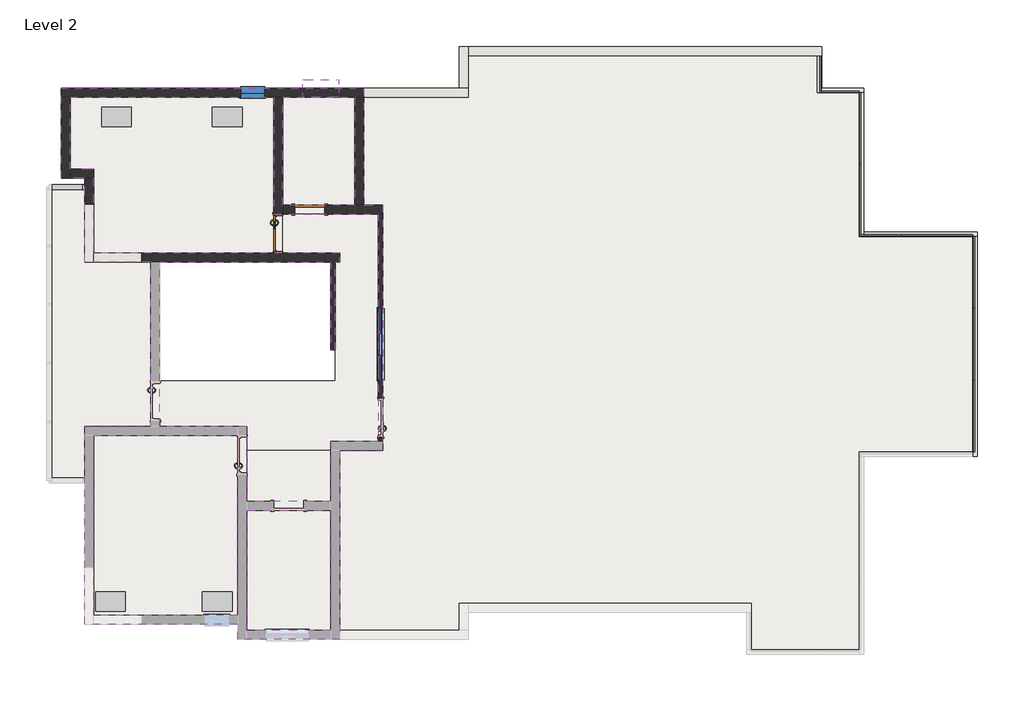
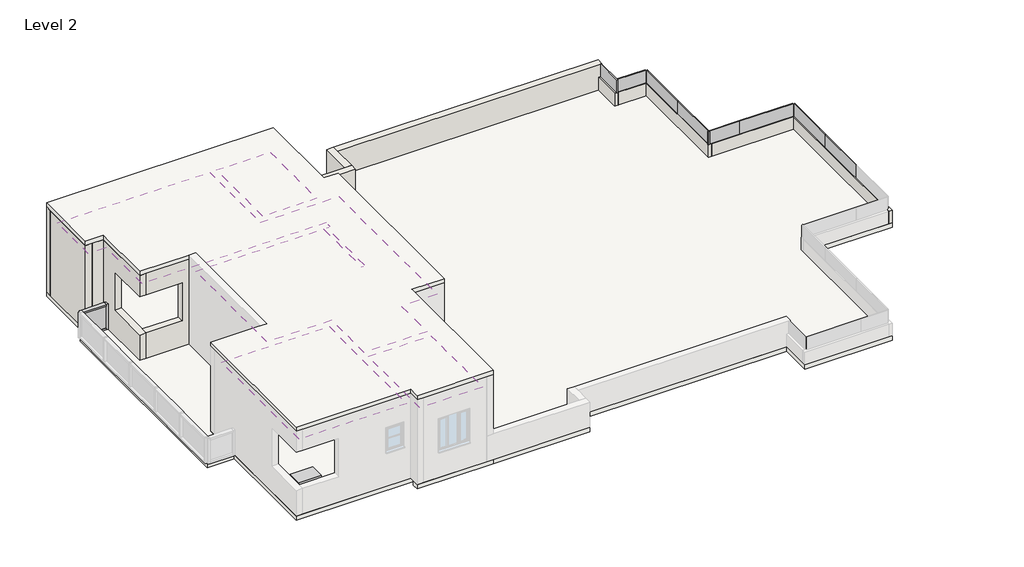
# One storey, part 2 of 2: 18 walls, 9 plates, 8 slabs, 4 coverings, 4 furniture elements, 3 members, 3 windows, 2 doors.
"""IFC4 building model written with IfcOpenShell, lengths in millimetres."""

from ifc_helpers import new_model, si_unit, frame, origin, place, context, project, spatial, polyline, outline, extrude, faceted_brep, transform, mapped, element, save
from components import door_cca51ba5, door_85036156, furniture_cabinet_file_lateral_3_drawer_760_x_500_x_915mm_92c95d2d, furniture_cabinet_file_lateral_3_drawer_760_x_500_x_915mm_e725971a, member_429f6687, member_73c23c35, system_panel_glazed_cc3a876e, system_panel_glazed_f05af352, system_panel_glazed_20ce4246, system_panel_glazed_67d0ec78, system_panel_glazed_26639370, fixed_ven_3_x1_1ea7015b, windows_sgl_swept_head_window_2_x3_cc7253b0, windows_tpl_plain_window_6_x4_c470b90d

model = new_model("IFC4")

# Units and contexts
model_context = context("Model", 3, world=origin())
ifc_project = project(units=[si_unit("LENGTHUNIT", "METRE", prefix="MILLI")], contexts=[model_context])

# Site, building, storey
site = spatial("IfcSite", under=ifc_project)
building = spatial("IfcBuilding", under=site)
storey = spatial("IfcBuildingStorey", under=building, Name="Level 2", Elevation=3200.4)

# Coverings
placement = place(None, origin())
element("IfcCovering", 1, ObjectType="2' x 4' ACT System", at=placement, inside=storey, context=model_context, shape_type="SweptSolid", body=[
    extrude(outline(polyline([(-7484.2378503, 5813.5135417), (-7484.2378503, 7642.3135417), (-2302.6378503, 7642.3135417), (-2302.6378503, 4670.5135417), (364.3621497, 4670.5135417), (364.3621497, -1120.6864583), (-854.8378503, -1120.6864583), (-854.8378503, -2644.7648645), (-2988.4378503, -2644.7648645), (-2988.4378503, -739.6864583), (-5197.7457903, -739.6864583), (-5197.7457903, 3451.3135417), (-854.8378503, 3451.3135417), (-854.8378503, 1216.1135417), (-740.5378503, 1216.1135417), (-740.5378503, 3451.3135417), (-626.2378503, 3451.3135417), (-626.2378503, 3679.9135417), (-6874.6378503, 3679.9135417), (-6874.6378503, 5813.5135417), (-7484.2378503, 5813.5135417)])), frame((0.0, 0.0, 5740.4), z_axis=(0.0, 0.0, 1.0), x_axis=(1.0, 0.0, 0.0)), (0.0, 0.0, 1.0), 57.15),
])
element("IfcCovering", 2, ObjectType="2' x 4' ACT System", at=placement, inside=storey, context=model_context, shape_type="SweptSolid", body=[
    extrude(outline(polyline([(-2074.0378503, 7642.3135417), (-245.2378503, 7642.3135417), (-245.2378503, 4899.1135417), (-2074.0378503, 4899.1135417), (-2074.0378503, 7642.3135417)])), frame((0.0, 0.0, 5740.4), z_axis=(0.0, 0.0, 1.0), x_axis=(1.0, 0.0, 0.0)), (0.0, 0.0, 1.0), 57.15),
])
element("IfcCovering", 3, ObjectType="2' x 4' ACT System", at=placement, inside=storey, context=model_context, shape_type="SweptSolid", body=[
    extrude(outline(polyline([(-6874.6378503, -5540.2864583), (-6874.6378503, -968.2864583), (-3217.0378503, -968.2864583), (-3217.0378503, -5540.2864583), (-6874.6378503, -5540.2864583)])), frame((0.0, 0.0, 5740.4), z_axis=(0.0, 0.0, 1.0), x_axis=(1.0, 0.0, 0.0)), (0.0, 0.0, 1.0), 57.15),
])
element("IfcCovering", 4, ObjectType="2' x 4' ACT System", at=placement, inside=storey, context=model_context, shape_type="SweptSolid", body=[
    extrude(outline(polyline([(-2988.4378503, -5921.3648645), (-2988.4378503, -2873.3648645), (-854.8378503, -2873.3648645), (-854.8378503, -5921.3648645), (-2988.4378503, -5921.3648645)])), frame((0.0, 0.0, 5740.4), z_axis=(0.0, 0.0, 1.0), x_axis=(1.0, 0.0, 0.0)), (0.0, 0.0, 1.0), 57.15),
])

# Doors
door_shape = door_cca51ba5(model_context)
element("IfcDoor", 5, ObjectType="Doors_IntSgl_4 : Internal Door 3'3\"X7'", at=placement, inside=storey, context=model_context, shape_type="MappedRepresentation", body=[
    mapped(door_shape, transform((-2188.3378503, 4175.2135417, 3200.4), x_axis=(0.0, -1.0, 0.0), y_axis=(1.0, 0.0, 0.0), z_axis=(0.0, 0.0, 1.0))),
])
door_2_shape = door_85036156(model_context)
element("IfcDoor", 6, ObjectType="Single-Flush : 2'6\"", at=placement, inside=storey, context=model_context, shape_type="MappedRepresentation", body=[
    mapped(door_2_shape, transform((-1388.2378503, 4784.8135417, 3200.4), x_axis=(-1.0, 0.0, 0.0), y_axis=(0.0, -1.0, 0.0), z_axis=(0.0, 0.0, 1.0))),
])

# Furniture
furniture_cabinet_file_lateral_3_drawer_760_x_500_x_915mm_shape = furniture_cabinet_file_lateral_3_drawer_760_x_500_x_915mm_92c95d2d(model_context)
element("IfcFurniture", 7, ObjectType="Furniture_Cabinet_File_Lateral_3-Drawer : 760 x 500 x 915mm", at=placement, inside=storey, context=model_context, shape_type="MappedRepresentation", body=[
    mapped(furniture_cabinet_file_lateral_3_drawer_760_x_500_x_915mm_shape, transform((-6122.6232763, 8081.3319178, 3200.4), x_axis=(1.0, 0.0, 0.0), y_axis=(0.0, 1.0, 0.0), z_axis=(0.0, 0.0, 1.0))),
])
element("IfcFurniture", 8, ObjectType="Furniture_Cabinet_File_Lateral_3-Drawer : 760 x 500 x 915mm", at=placement, inside=storey, context=model_context, shape_type="MappedRepresentation", body=[
    mapped(furniture_cabinet_file_lateral_3_drawer_760_x_500_x_915mm_shape, transform((-3303.7153364, 8081.3319178, 3200.4), x_axis=(1.0, 0.0, 0.0), y_axis=(0.0, 1.0, 0.0), z_axis=(0.0, 0.0, 1.0))),
])
furniture_cabinet_file_lateral_3_drawer_760_x_500_x_915mm_2_shape = furniture_cabinet_file_lateral_3_drawer_760_x_500_x_915mm_e725971a(model_context)
element("IfcFurniture", 9, ObjectType="Furniture_Cabinet_File_Lateral_3-Drawer : 760 x 500 x 915mm", at=placement, inside=storey, context=model_context, shape_type="MappedRepresentation", body=[
    mapped(furniture_cabinet_file_lateral_3_drawer_760_x_500_x_915mm_2_shape, transform((-3557.7153364, -6131.7832406, 3200.4), x_axis=(1.0, 0.0, 0.0), y_axis=(0.0, 1.0, 0.0), z_axis=(0.0, 0.0, 1.0))),
])
element("IfcFurniture", 10, ObjectType="Furniture_Cabinet_File_Lateral_3-Drawer : 760 x 500 x 915mm", at=placement, inside=storey, context=model_context, shape_type="MappedRepresentation", body=[
    mapped(furniture_cabinet_file_lateral_3_drawer_760_x_500_x_915mm_2_shape, transform((-6275.5153364, -6131.7832406, 3200.4), x_axis=(1.0, 0.0, 0.0), y_axis=(0.0, 1.0, 0.0), z_axis=(0.0, 0.0, 1.0))),
])

# Members
member_shape = member_429f6687(model_context)
element("IfcMember", 11, ObjectType="Rectangular Mullion : 2.5\" x 5\" rectangular", at=placement, inside=storey, context=model_context, shape_type="MappedRepresentation", body=[
    mapped(member_shape, transform((-7954.1378503, 5356.1494886, 4114.8), x_axis=(0.0, 0.0, 1.0), y_axis=(0.0, 1.0, 0.0), z_axis=(-1.0, 0.0, 0.0))),
])
element("IfcMember", 12, ObjectType="Rectangular Mullion : 2.5\" x 5\" rectangular", at=placement, inside=storey, context=model_context, shape_type="MappedRepresentation", body=[
    mapped(member_shape, transform((-7166.7378503, 5356.1494886, 3200.4), x_axis=(0.0, 0.0, -1.0), y_axis=(0.0, 1.0, 0.0), z_axis=(1.0, 0.0, 0.0))),
])
member_2_shape = member_73c23c35(model_context)
element("IfcMember", 13, ObjectType="Rectangular Mullion : 2.5\" x 5\" rectangular", at=placement, inside=storey, context=model_context, shape_type="MappedRepresentation", body=[
    mapped(member_2_shape, transform((-7103.2378503, 5356.1494886, 4114.8), x_axis=(1.0, 0.0, 0.0), y_axis=(0.0, 1.0, 0.0), z_axis=(0.0, 0.0, 1.0))),
])

# Plates
system_panel_glazed_shape = system_panel_glazed_cc3a876e(model_context)
element("IfcPlate", 14, ObjectType="System Panel : Glazed", at=placement, inside=storey, context=model_context, shape_type="MappedRepresentation", body=[
    mapped(system_panel_glazed_shape, transform((12118.2121497, 7756.6135417, 3657.6), x_axis=(-1.0, 0.0, 0.0), y_axis=(0.0, -1.0, 0.0), z_axis=(0.0, 0.0, 1.0))),
])
system_panel_glazed_2_shape = system_panel_glazed_f05af352(model_context)
element("IfcPlate", 15, ObjectType="System Panel : Glazed", at=placement, inside=storey, context=model_context, shape_type="MappedRepresentation", body=[
    mapped(system_panel_glazed_2_shape, transform((15490.0621497, 1355.813542, 3657.6), x_axis=(0.0, 1.0, 0.0), y_axis=(-1.0, 0.0, 0.0), z_axis=(0.0, 0.0, 1.0))),
])
element("IfcPlate", 16, ObjectType="System Panel : Glazed", at=placement, inside=storey, context=model_context, shape_type="MappedRepresentation", body=[
    mapped(system_panel_glazed_2_shape, transform((15490.0621497, 3184.6135419, 3657.6), x_axis=(0.0, 1.0, 0.0), y_axis=(-1.0, 0.0, 0.0), z_axis=(0.0, 0.0, 1.0))),
])
element("IfcPlate", 17, ObjectType="System Panel : Glazed", at=placement, inside=storey, context=model_context, shape_type="MappedRepresentation", body=[
    mapped(system_panel_glazed_2_shape, transform((14575.6621496, 4099.0135417, 3657.6), x_axis=(-1.0, 0.0, 0.0), y_axis=(0.0, -1.0, 0.0), z_axis=(0.0, 0.0, 1.0))),
])
element("IfcPlate", 18, ObjectType="System Panel : Glazed", at=placement, inside=storey, context=model_context, shape_type="MappedRepresentation", body=[
    mapped(system_panel_glazed_2_shape, transform((12594.4621497, 5013.4135419, 3657.6), x_axis=(0.0, 1.0, 0.0), y_axis=(-1.0, 0.0, 0.0), z_axis=(0.0, 0.0, 1.0))),
])
element("IfcPlate", 19, ObjectType="System Panel : Glazed", at=placement, inside=storey, context=model_context, shape_type="MappedRepresentation", body=[
    mapped(system_panel_glazed_2_shape, transform((12594.4621497, 6842.2135419, 3657.6), x_axis=(0.0, 1.0, 0.0), y_axis=(-1.0, 0.0, 0.0), z_axis=(0.0, 0.0, 1.0))),
])
system_panel_glazed_3_shape = system_panel_glazed_20ce4246(model_context)
element("IfcPlate", 20, ObjectType="System Panel : Glazed", at=placement, inside=storey, context=model_context, shape_type="MappedRepresentation", body=[
    mapped(system_panel_glazed_3_shape, transform((13127.8621496, 4099.0135417, 3657.6), x_axis=(-1.0, 0.0, 0.0), y_axis=(0.0, -1.0, 0.0), z_axis=(0.0, 0.0, 1.0))),
])
system_panel_glazed_4_shape = system_panel_glazed_67d0ec78(model_context)
element("IfcPlate", 21, ObjectType="System Panel : Glazed", at=placement, inside=storey, context=model_context, shape_type="MappedRepresentation", body=[
    mapped(system_panel_glazed_4_shape, transform((11641.9621497, 8232.8635417, 3657.6), x_axis=(0.0, 1.0, 0.0), y_axis=(-1.0, 0.0, 0.0), z_axis=(0.0, 0.0, 1.0))),
])
system_panel_glazed_5_shape = system_panel_glazed_26639370(model_context)
element("IfcPlate", 22, ObjectType="System Panel : Glazed", at=placement, inside=storey, context=model_context, shape_type="MappedRepresentation", body=[
    mapped(system_panel_glazed_5_shape, transform((-7560.4378503, 5356.1494886, 3263.9), x_axis=(-1.0, 0.0, 0.0), y_axis=(0.0, -1.0, 0.0), z_axis=(0.0, 0.0, 1.0))),
])

# Slabs
element("IfcSlab", 23, ObjectType="Generic - 6\"", at=placement, inside=storey, context=model_context, shape_type="SweptSolid", body=[
    extrude(outline(polyline([(-16.6378503, 7870.9135417), (2421.7621497, 7870.9135417), (2421.7621497, 8937.7135417), (11641.9621497, 8937.7135417), (11641.9621497, 7870.9135417), (12708.7621497, 7870.9135417), (12708.7621497, 4213.3135417), (15604.3621497, 4213.3135417), (15604.3621497, -1501.6864583), (12708.7621497, -1501.6864583), (12708.7621497, -6530.8864583), (9736.9621497, -6530.8864583), (9736.9621497, -5464.0864583), (2650.3621497, -5464.0864583), (2650.3621497, -6149.9648645), (-626.2378503, -6149.9648645), (-626.2378503, -5921.3648645), (-626.2378503, -1349.2864583), (478.6621497, -1349.2864583), (478.6621497, 4899.1135417), (-16.6378503, 4899.1135417), (-16.6378503, 7870.9135417)])), frame((0.0, 0.0, 3048.0), z_axis=(0.0, 0.0, 1.0), x_axis=(1.0, 0.0, 0.0)), (0.0, 0.0, 1.0), 152.4),
])
element("IfcSlab", 24, ObjectType="Generic - 6\"", at=placement, inside=storey, context=model_context, shape_type="SweptSolid", body=[
    extrude(outline(polyline([(-2988.4378503, -739.6864583), (-2988.4378503, -5768.9648645), (-7103.2378503, -5768.9648645), (-7103.2378503, -739.6864583), (-2988.4378503, -739.6864583)])), frame((0.0, 0.0, 3048.0), z_axis=(0.0, 0.0, 1.0), x_axis=(1.0, 0.0, 0.0)), (0.0, 0.0, 1.0), 152.4),
])
element("IfcSlab", 25, ObjectType="Generic - 6\"", at=placement, inside=storey, context=model_context, shape_type="SweptSolid", body=[
    extrude(outline(polyline([(-3217.0378503, -5921.3648645), (-2988.4378503, -5921.3648645), (-2988.4378503, -1349.2864583), (-626.2378503, -1349.2864583), (-626.2378503, -6149.9648645), (-3217.0378503, -6149.9648645), (-3217.0378503, -5921.3648645)])), frame((0.0, 0.0, 3048.0), z_axis=(0.0, 0.0, 1.0), x_axis=(1.0, 0.0, 0.0)), (0.0, 0.0, 1.0), 152.4),
])
element("IfcSlab", 26, ObjectType="Generic - 6\"", at=placement, inside=storey, context=model_context, shape_type="SweptSolid", body=[
    extrude(outline(polyline([(-8017.6378503, 5356.1494886), (-7103.2378503, 5356.1494886), (-7103.2378503, 3451.3135417), (-5426.3457903, 3451.3135417), (-5426.3457903, -739.6864583), (-7103.2378503, -739.6864583), (-7103.2378503, -2111.2864583), (-8017.6378503, -2111.2864583), (-8017.6378503, 5356.1494886)])), frame((0.0, 0.0, 3048.0), z_axis=(0.0, 0.0, 1.0), x_axis=(1.0, 0.0, 0.0)), (0.0, 0.0, 1.0), 152.4),
])
element("IfcSlab", 27, ObjectType="Generic - 6\"", at=placement, inside=storey, context=model_context, shape_type="SweptSolid", body=[
    extrude(outline(polyline([(-2302.6378503, 7870.9135417), (-16.6378503, 7870.9135417), (-16.6378503, 4670.5135417), (-2302.6378503, 4670.5135417), (-2302.6378503, 7870.9135417)])), frame((0.0, 0.0, 3048.0), z_axis=(0.0, 0.0, 1.0), x_axis=(1.0, 0.0, 0.0)), (0.0, 0.0, 1.0), 152.4),
])
element("IfcSlab", 28, ObjectType="Generic - 6\"", at=placement, inside=storey, context=model_context, shape_type="SweptSolid", body=[
    extrude(outline(polyline([(-7712.8378503, 7870.9135417), (-2302.6378503, 7870.9135417), (-2302.6378503, 4670.5135417), (-2074.0378503, 4670.5135417), (-2074.0378503, 3451.3135417), (-7103.2378503, 3451.3135417), (-7103.2378503, 5584.9135417), (-7712.8378503, 5584.9135417), (-7712.8378503, 7870.9135417)])), frame((0.0, 0.0, 3048.0), z_axis=(0.0, 0.0, 1.0), x_axis=(1.0, 0.0, 0.0)), (0.0, 0.0, 1.0), 152.4),
])
element("IfcSlab", 29, ObjectType="Generic - 6\"", at=placement, inside=storey, context=model_context, shape_type="SweptSolid", body=[
    extrude(outline(polyline([(478.6621497, 4899.1135417), (478.6621497, -1349.2864583), (-2988.4378503, -1349.2864583), (-2988.4378503, -739.6864583), (-5426.3457903, -739.6864583), (-5426.3457903, 3451.3135417), (-5197.7457903, 3451.3135417), (-5197.7457903, 416.1965995), (-740.5378503, 416.1965995), (-740.5378503, 3451.3135417), (-2074.0378503, 3451.3135417), (-2074.0378503, 4670.5135417), (-16.6378503, 4670.5135417), (-16.6378503, 4899.1135417), (478.6621497, 4899.1135417)])), frame((0.0, 0.0, 3048.0), z_axis=(0.0, 0.0, 1.0), x_axis=(1.0, 0.0, 0.0)), (0.0, 0.0, 1.0), 152.4),
])
element("IfcSlab", 30, ObjectType="Generic - 6\"", at=placement, inside=storey, context=model_context, shape_type="SweptSolid", body=[
    extrude(outline(polyline([(-16.6378503, 7870.9135417), (-16.6378503, 4899.1135417), (478.6621497, 4899.1135417), (478.6621497, -1349.2864583), (-626.2378503, -1349.2864583), (-626.2378503, -6149.9648645), (-3217.0378503, -6149.9648645), (-3217.0378503, -5768.8864583), (-7103.2378503, -5768.8864583), (-7103.2378503, -739.6864583), (-5426.3457903, -739.6864583), (-5426.3457903, 3451.3135417), (-7103.2378503, 3451.3135417), (-7103.2378503, 5584.9135417), (-7712.8378503, 5584.9135417), (-7712.8378503, 7870.9135417), (-16.6378503, 7870.9135417)])), frame((0.0, 0.0, 6248.4), z_axis=(0.0, 0.0, 1.0), x_axis=(1.0, 0.0, 0.0)), (0.0, 0.0, 1.0), 152.4),
])

# Walls
element("IfcWall", 31, ObjectType="Generic - 4.5\"", at=placement, inside=storey, context=model_context, shape_type="Brep", body=[
    faceted_brep([(11527.6621497, 8709.1135417, 3200.4), (11527.6621497, 7756.6135417, 3200.4), (11527.6621497, 7756.6135417, 3657.6), (11527.6621497, 8709.1135417, 3657.6), (11641.9621497, 8709.1135417, 3200.4), (11641.9621497, 8709.1135417, 3657.6), (11641.9621497, 7870.9135417, 3657.6), (11641.9621497, 7756.6135417, 3657.6), (11641.9621497, 7756.6135417, 3200.4), (11641.9621497, 7870.9135417, 3200.4)], [[[0, 1, 2, 3]], [[4, 5, 6, 7, 8, 9]], [[1, 0, 4, 9, 8]], [[3, 2, 7, 6, 5]], [[0, 3, 5, 4]], [[2, 1, 8, 7]]]),
])
element("IfcWall", 32, ObjectType="Generic - 4.5\"", at=placement, inside=storey, context=model_context, shape_type="Brep", body=[
    faceted_brep([(11641.9621497, 7756.6135417, 3200.4), (12594.4621497, 7756.6135417, 3200.4), (12708.7621497, 7756.6135417, 3200.4), (12708.7621497, 7756.6135417, 3657.6), (12594.4621497, 7756.6135417, 3657.6), (11641.9621497, 7756.6135417, 3657.6), (11641.9621497, 7870.9135417, 3200.4), (11641.9621497, 7870.9135417, 3657.6), (12708.7621497, 7870.9135417, 3657.6), (12708.7621497, 7870.9135417, 3200.4)], [[[0, 1, 2, 3, 4, 5]], [[6, 7, 8, 9]], [[2, 1, 0, 6, 9]], [[5, 4, 3, 8, 7]], [[0, 5, 7, 6]], [[3, 2, 9, 8]]]),
])
element("IfcWall", 33, ObjectType="Generic - 4.5\"", at=placement, inside=storey, context=model_context, shape_type="Brep", body=[
    faceted_brep([(12594.4621497, 7756.6135417, 3200.4), (12594.4621497, 4099.0135417, 3200.4), (12594.4621497, 4099.0135417, 3657.6), (12594.4621497, 7756.6135417, 3657.6), (12708.7621497, 7756.6135417, 3200.4), (12708.7621497, 7756.6135417, 3657.6), (12708.7621497, 4213.3135417, 3657.6), (12708.7621497, 4099.0135417, 3657.6), (12708.7621497, 4099.0135417, 3200.4), (12708.7621497, 4213.3135417, 3200.4)], [[[0, 1, 2, 3]], [[4, 5, 6, 7, 8, 9]], [[1, 0, 4, 9, 8]], [[3, 2, 7, 6, 5]], [[0, 3, 5, 4]], [[2, 1, 8, 7]]]),
])
element("IfcWall", 34, ObjectType="Generic - 4.5\"", at=placement, inside=storey, context=model_context, shape_type="Brep", body=[
    faceted_brep([(12708.7621497, 4099.0135417, 3200.4), (15490.0621497, 4099.0135417, 3200.4), (15604.3621497, 4099.0135417, 3200.4), (15604.3621497, 4099.0135417, 3657.6), (15490.0621497, 4099.0135417, 3657.6), (12708.7621497, 4099.0135417, 3657.6), (12708.7621497, 4213.3135417, 3200.4), (12708.7621497, 4213.3135417, 3657.6), (15604.3621497, 4213.3135417, 3657.6), (15604.3621497, 4213.3135417, 3200.4)], [[[0, 1, 2, 3, 4, 5]], [[6, 7, 8, 9]], [[2, 1, 0, 6, 9]], [[5, 4, 3, 8, 7]], [[0, 5, 7, 6]], [[3, 2, 9, 8]]]),
])
element("IfcWall", 35, ObjectType="Generic - 4.5\"", at=placement, inside=storey, context=model_context, shape_type="Brep", body=[
    faceted_brep([(15490.0621497, 4099.0135417, 3200.4), (15490.0621497, -1387.3864583, 3200.4), (15490.0621497, -1501.6864583, 3200.4), (15490.0621497, -1501.6864583, 3657.6), (15490.0621497, -1387.3864583, 3657.6), (15490.0621497, 4099.0135417, 3657.6), (15604.3621497, 4099.0135417, 3200.4), (15604.3621497, 4099.0135417, 3657.6), (15604.3621497, -1501.6864583, 3657.6), (15604.3621497, -1501.6864583, 3200.4)], [[[0, 1, 2, 3, 4, 5]], [[6, 7, 8, 9]], [[2, 1, 0, 6, 9]], [[5, 4, 3, 8, 7]], [[0, 5, 7, 6]], [[3, 2, 9, 8]]]),
])
element("IfcWall", 36, ObjectType="Generic - 4.5\"", at=placement, inside=storey, context=model_context, shape_type="SweptSolid", body=[
    extrude(outline(polyline([(4670.5135417, 6248.4), (4670.5135417, 3200.4), (-15.7864583, 3200.4), (-15.7864583, 5334.0), (-1006.3864583, 5334.0), (-1006.3864583, 3200.4), (-1120.6864583, 3200.4), (-1120.6864583, 6248.4), (4670.5135417, 6248.4)]), holes=[polyline([(2270.2135417, 5310.4), (441.4135417, 5310.4), (441.4135417, 4091.2), (2270.2135417, 4091.2), (2270.2135417, 5310.4)])]), frame((364.3621497, 0.0, 0.0), z_axis=(1.0, 0.0, 0.0), x_axis=(0.0, 1.0, 0.0)), (0.0, 0.0, 1.0), 114.3),
])
element("IfcWall", 37, ObjectType="Generic - 4.5\"", at=placement, inside=storey, context=model_context, shape_type="SweptSolid", body=[
    extrude(outline(polyline([(-854.8378503, 1216.1135417), (-854.8378503, 3451.3135417), (-740.5378503, 3451.3135417), (-740.5378503, 1216.1135417), (-854.8378503, 1216.1135417)])), frame((0.0, 0.0, 3200.4), z_axis=(0.0, 0.0, 1.0), x_axis=(1.0, 0.0, 0.0)), (0.0, 0.0, 1.0), 3048.0),
])
element("IfcWall", 38, ObjectType="Generic - 9\"", at=placement, inside=storey, context=model_context, shape_type="Brep", body=[
    faceted_brep([(-16.6378503, 7642.3135417, 3200.4), (2650.3621497, 7642.3135417, 3200.4), (2650.3621497, 7642.3135417, 4114.8), (-16.6378503, 7642.3135417, 4114.8), (-16.6378503, 7870.9135417, 3200.4), (-16.6378503, 7870.9135417, 4114.8), (2421.7621497, 7870.9135417, 4114.8), (2650.3621497, 7870.9135417, 4114.8), (2650.3621497, 7870.9135417, 3200.4), (2421.7621497, 7870.9135417, 3200.4)], [[[0, 1, 2, 3]], [[4, 5, 6, 7, 8, 9]], [[1, 0, 4, 9, 8]], [[3, 2, 7, 6, 5]], [[2, 1, 8, 7]], [[0, 3, 5, 4]]]),
])
element("IfcWall", 39, ObjectType="Generic - 9\"", at=placement, inside=storey, context=model_context, shape_type="Brep", body=[
    faceted_brep([(2650.3621497, 7870.9135417, 3200.4), (2650.3621497, 8709.1135417, 3200.4), (2650.3621497, 8937.7135417, 3200.4), (2650.3621497, 8937.7135417, 4114.8), (2650.3621497, 8709.1135417, 4114.8), (2650.3621497, 7870.9135417, 4114.8), (2421.7621497, 7870.9135417, 3200.4), (2421.7621497, 7870.9135417, 4114.8), (2421.7621497, 8937.7135417, 4114.8), (2421.7621497, 8937.7135417, 3200.4)], [[[0, 1, 2, 3, 4, 5]], [[6, 7, 8, 9]], [[2, 1, 0, 6, 9]], [[5, 4, 3, 8, 7]], [[0, 5, 7, 6]], [[3, 2, 9, 8]]]),
])
element("IfcWall", 40, ObjectType="Generic - 9\"", at=placement, inside=storey, context=model_context, shape_type="Brep", body=[
    faceted_brep([(2650.3621497, 8709.1135417, 3200.4), (11527.6621497, 8709.1135417, 3200.4), (11641.9621497, 8709.1135417, 3200.4), (11641.9621497, 8709.1135417, 3657.6), (11641.9621497, 8709.1135417, 4114.8), (2650.3621497, 8709.1135417, 4114.8), (2650.3621497, 8937.7135417, 3200.4), (2650.3621497, 8937.7135417, 4114.8), (11641.9621497, 8937.7135417, 4114.8), (11641.9621497, 8937.7135417, 3200.4)], [[[0, 1, 2, 3, 4, 5]], [[6, 7, 8, 9]], [[2, 1, 0, 6, 9]], [[5, 4, 8, 7]], [[0, 5, 7, 6]], [[4, 3, 2, 9, 8]]]),
])
element("IfcWall", 41, ObjectType="Generic - 9\"", at=placement, inside=storey, context=model_context, shape_type="Brep", body=[
    faceted_brep([(-7712.8378503, 7642.3135417, 3200.4), (-7484.2378503, 7642.3135417, 3200.4), (-2302.6378503, 7642.3135417, 3200.4), (-2074.0378503, 7642.3135417, 3200.4), (-245.2378503, 7642.3135417, 3200.4), (-16.6378503, 7642.3135417, 3200.4), (-16.6378503, 7642.3135417, 4114.8), (-16.6378503, 7642.3135417, 6248.4), (-245.2378503, 7642.3135417, 6248.4), (-2074.0378503, 7642.3135417, 6248.4), (-2302.6378503, 7642.3135417, 6248.4), (-7484.2378503, 7642.3135417, 6248.4), (-7712.8378503, 7642.3135417, 6248.4), (-1559.6878503, 7642.3135417, 5638.8), (-645.2878503, 7642.3135417, 5638.8), (-645.2878503, 7642.3135417, 5334.0), (-1559.6878503, 7642.3135417, 5334.0), (-3140.8378503, 7642.3135417, 5310.4), (-2531.2378503, 7642.3135417, 5310.4), (-2531.2378503, 7642.3135417, 4396.0), (-3140.8378503, 7642.3135417, 4396.0), (-7712.8378503, 7870.9135417, 3200.4), (-7712.8378503, 7870.9135417, 6248.4), (-16.6378503, 7870.9135417, 6248.4), (-16.6378503, 7870.9135417, 4114.8), (-16.6378503, 7870.9135417, 3200.4), (-1559.6878503, 7870.9135417, 5638.8), (-1559.6878503, 7870.9135417, 5334.0), (-645.2878503, 7870.9135417, 5334.0), (-645.2878503, 7870.9135417, 5638.8), (-3140.8378503, 7870.9135417, 5310.4), (-3140.8378503, 7870.9135417, 4396.0), (-2531.2378503, 7870.9135417, 4396.0), (-2531.2378503, 7870.9135417, 5310.4)], [[[0, 1, 2, 3, 4, 5, 6, 7, 8, 9, 10, 11, 12], [13, 14, 15, 16], [17, 18, 19, 20]], [[21, 22, 23, 24, 25], [26, 27, 28, 29], [30, 31, 32, 33]], [[5, 4, 3, 2, 1, 0, 21, 25]], [[5, 25, 24, 23, 7, 6]], [[0, 12, 22, 21]], [[27, 26, 13, 16]], [[28, 27, 16, 15]], [[29, 28, 15, 14]], [[26, 29, 14, 13]], [[31, 30, 17, 20]], [[32, 31, 20, 19]], [[33, 32, 19, 18]], [[30, 33, 18, 17]], [[12, 11, 10, 9, 8, 7, 23, 22]]]),
])
element("IfcWall", 42, ObjectType="Generic - 9\"", at=placement, inside=storey, context=model_context, shape_type="SweptSolid", body=[
    extrude(outline(polyline([(-245.2378503, 4899.1135417), (-245.2378503, 7642.3135417), (-16.6378503, 7642.3135417), (-16.6378503, 4899.1135417), (-245.2378503, 4899.1135417)])), frame((0.0, 0.0, 3200.4), z_axis=(0.0, 0.0, 1.0), x_axis=(1.0, 0.0, 0.0)), (0.0, 0.0, 1.0), 3048.0),
])
element("IfcWall", 43, ObjectType="Generic - 9\"", at=placement, inside=storey, context=model_context, shape_type="Brep", body=[
    faceted_brep([(-1769.2378503, 4899.1135417, 5232.4), (-1769.2378503, 4899.1135417, 3200.4), (-2074.0378503, 4899.1135417, 3200.4), (-2074.0378503, 4899.1135417, 6248.4), (-245.2378503, 4899.1135417, 6248.4), (-16.6378503, 4899.1135417, 6248.4), (478.6621497, 4899.1135417, 6248.4), (478.6621497, 4899.1135417, 3200.4), (-16.6378503, 4899.1135417, 3200.4), (-245.2378503, 4899.1135417, 3200.4), (-1007.2378503, 4899.1135417, 3200.4), (-1007.2378503, 4899.1135417, 5232.4), (-2074.0378503, 4670.5135417, 3200.4), (-1769.2378503, 4670.5135417, 3200.4), (-1769.2378503, 4670.5135417, 5232.4), (-1007.2378503, 4670.5135417, 5232.4), (-1007.2378503, 4670.5135417, 3200.4), (364.3621497, 4670.5135417, 3200.4), (478.6621497, 4670.5135417, 3200.4), (478.6621497, 4670.5135417, 6248.4), (364.3621497, 4670.5135417, 6248.4), (-2074.0378503, 4670.5135417, 6248.4)], [[[0, 1, 2, 3, 4, 5, 6, 7, 8, 9, 10, 11]], [[12, 13, 14, 15, 16, 17, 18, 19, 20, 21]], [[2, 1, 13, 12]], [[10, 9, 8, 7, 18, 17, 16]], [[7, 6, 19, 18]], [[3, 2, 12, 21]], [[14, 13, 1, 0]], [[15, 14, 0, 11]], [[16, 15, 11, 10]], [[6, 5, 4, 3, 21, 20, 19]]]),
])
element("IfcWall", 44, ObjectType="Generic - 9\"", at=placement, inside=storey, context=model_context, shape_type="Brep", body=[
    faceted_brep([(-2074.0378503, 7642.3135417, 3200.4), (-2074.0378503, 7642.3135417, 6248.4), (-2074.0378503, 4899.1135417, 6248.4), (-2074.0378503, 4670.5135417, 6248.4), (-2074.0378503, 3679.9135417, 6248.4), (-2074.0378503, 3679.9135417, 5334.0), (-2074.0378503, 4670.5135417, 5334.0), (-2074.0378503, 4670.5135417, 3200.4), (-2074.0378503, 4899.1135417, 3200.4), (-2302.6378503, 7642.3135417, 6248.4), (-2302.6378503, 7642.3135417, 3200.4), (-2302.6378503, 4670.5135417, 3200.4), (-2302.6378503, 4670.5135417, 5334.0), (-2302.6378503, 3679.9135417, 5334.0), (-2302.6378503, 3679.9135417, 6248.4)], [[[0, 1, 2, 3, 4, 5, 6, 7, 8]], [[9, 10, 11, 12, 13, 14]], [[10, 0, 8, 7, 11]], [[1, 0, 10, 9]], [[4, 14, 13, 5]], [[12, 6, 5, 13]], [[6, 12, 11, 7]], [[4, 3, 2, 1, 9, 14]]]),
])
element("IfcWall", 45, ObjectType="Generic - 9\"", at=placement, inside=storey, context=model_context, shape_type="Brep", body=[
    faceted_brep([(-7712.8378503, 7642.3135417, 3200.4), (-7712.8378503, 5584.9135417, 3200.4), (-7712.8378503, 5584.9135417, 6248.4), (-7712.8378503, 7642.3135417, 6248.4), (-7484.2378503, 7642.3135417, 3200.4), (-7484.2378503, 7642.3135417, 6248.4), (-7484.2378503, 5813.5135417, 6248.4), (-7484.2378503, 5584.9135417, 6248.4), (-7484.2378503, 5584.9135417, 3200.4), (-7484.2378503, 5813.5135417, 3200.4)], [[[0, 1, 2, 3]], [[4, 5, 6, 7, 8, 9]], [[1, 0, 4, 9, 8]], [[0, 3, 5, 4]], [[2, 1, 8, 7]], [[3, 2, 7, 6, 5]]]),
])
element("IfcWall", 46, ObjectType="Generic - 9\"", at=placement, inside=storey, context=model_context, shape_type="Brep", body=[
    faceted_brep([(-7484.2378503, 5584.9135417, 3200.4), (-7103.2378503, 5584.9135417, 3200.4), (-6874.6378503, 5584.9135417, 3200.4), (-6874.6378503, 5584.9135417, 6248.4), (-7103.2378503, 5584.9135417, 6248.4), (-7484.2378503, 5584.9135417, 6248.4), (-7484.2378503, 5813.5135417, 3200.4), (-7484.2378503, 5813.5135417, 6248.4), (-6874.6378503, 5813.5135417, 6248.4), (-6874.6378503, 5813.5135417, 3200.4)], [[[0, 1, 2, 3, 4, 5]], [[6, 7, 8, 9]], [[2, 1, 0, 6, 9]], [[0, 5, 7, 6]], [[3, 2, 9, 8]], [[5, 4, 3, 8, 7]]]),
])
element("IfcWall", 47, ObjectType="Generic - 9\"", at=placement, inside=storey, context=model_context, shape_type="Brep", body=[
    faceted_brep([(-7103.2378503, 5584.9135417, 3200.4), (-7103.2378503, 3451.3135417, 3200.4), (-7103.2378503, 3451.3135417, 4114.8), (-7103.2378503, 4919.1012615, 4114.8), (-7103.2378503, 4919.1012615, 5486.4), (-7103.2378503, 3451.3135417, 5486.4), (-7103.2378503, 3451.3135417, 6248.4), (-7103.2378503, 5584.9135417, 6248.4), (-6874.6378503, 3451.3135417, 3200.4), (-6874.6378503, 3679.9135417, 3200.4), (-6874.6378503, 5584.9135417, 3200.4), (-6874.6378503, 5584.9135417, 6248.4), (-6874.6378503, 3679.9135417, 6248.4), (-6874.6378503, 3451.3135417, 6248.4), (-6874.6378503, 3451.3135417, 5486.4), (-6874.6378503, 3679.9135417, 5486.4), (-6874.6378503, 4919.1012615, 5486.4), (-6874.6378503, 4919.1012615, 4114.8), (-6874.6378503, 3679.9135417, 4114.8), (-6874.6378503, 3451.3135417, 4114.8)], [[[0, 1, 2, 3, 4, 5, 6, 7]], [[8, 9, 10, 11, 12, 13, 14, 15, 16, 17, 18, 19]], [[1, 0, 10, 9, 8]], [[0, 7, 11, 10]], [[4, 16, 15, 14, 5]], [[17, 3, 2, 19, 18]], [[16, 4, 3, 17]], [[1, 8, 19, 2]], [[13, 6, 5, 14]], [[7, 6, 13, 12, 11]]]),
])
element("IfcWall", 48, ObjectType="Generic - 9\"", at=placement, inside=storey, context=model_context, shape_type="Brep", body=[
    faceted_brep([(-6874.6378503, 3451.3135417, 3200.4), (-5426.3457903, 3451.3135417, 3200.4), (-5197.7457903, 3451.3135417, 3200.4), (-854.8378503, 3451.3135417, 3200.4), (-740.5378503, 3451.3135417, 3200.4), (-626.2378503, 3451.3135417, 3200.4), (-626.2378503, 3451.3135417, 6248.4), (-740.5378503, 3451.3135417, 6248.4), (-854.8378503, 3451.3135417, 6248.4), (-5426.3457903, 3451.3135417, 6248.4), (-6874.6378503, 3451.3135417, 6248.4), (-6874.6378503, 3451.3135417, 5486.4), (-5660.4501867, 3451.3135417, 5486.4), (-5660.4501867, 3451.3135417, 4114.8), (-6874.6378503, 3451.3135417, 4114.8), (-626.2378503, 3679.9135417, 3200.4), (-6874.6378503, 3679.9135417, 3200.4), (-6874.6378503, 3679.9135417, 4114.8), (-5660.4501867, 3679.9135417, 4114.8), (-5660.4501867, 3679.9135417, 5486.4), (-6874.6378503, 3679.9135417, 5486.4), (-6874.6378503, 3679.9135417, 6248.4), (-2302.6378503, 3679.9135417, 6248.4), (-2074.0378503, 3679.9135417, 6248.4), (-626.2378503, 3679.9135417, 6248.4)], [[[0, 1, 2, 3, 4, 5, 6, 7, 8, 9, 10, 11, 12, 13, 14]], [[15, 16, 17, 18, 19, 20, 21, 22, 23, 24]], [[5, 4, 3, 2, 1, 0, 16, 15]], [[6, 5, 15, 24]], [[19, 12, 11, 20]], [[13, 18, 17, 14]], [[12, 19, 18, 13]], [[10, 21, 20, 11]], [[16, 0, 14, 17]], [[10, 9, 8, 7, 6, 24, 23, 22, 21]]]),
])

# Windows
fixed_ven_3_x1_shape = fixed_ven_3_x1_1ea7015b(model_context)
element("IfcWindow", 49, ObjectType="Fixed : Ven 3'X1'", at=placement, inside=storey, context=model_context, shape_type="MappedRepresentation", body=[
    mapped(fixed_ven_3_x1_shape, transform((-1140.5878503, 7756.6135417, 3200.4), x_axis=(-1.0, 0.0, 0.0), y_axis=(0.0, -1.0, 0.0), z_axis=(0.0, 0.0, 1.0))),
])
windows_sgl_swept_head_window_2_x3_shape = windows_sgl_swept_head_window_2_x3_cc7253b0(model_context)
element("IfcWindow", 50, ObjectType="Windows_Sgl_Swept_Head : Window 2'X3'", at=placement, inside=storey, context=model_context, shape_type="MappedRepresentation", body=[
    mapped(windows_sgl_swept_head_window_2_x3_shape, transform((-2836.0378503, 7748.1569739, 3200.4), x_axis=(1.0, 0.0, 0.0), y_axis=(0.0, 1.0, 0.0), z_axis=(0.0, 0.0, 1.0))),
])
windows_tpl_plain_window_6_x4_shape = windows_tpl_plain_window_6_x4_c470b90d(model_context)
element("IfcWindow", 51, ObjectType="Windows_Tpl_Plain : Window 6'X4'", at=placement, inside=storey, context=model_context, shape_type="MappedRepresentation", body=[
    mapped(windows_tpl_plain_window_6_x4_shape, transform((413.0555819, 776.0135417, 3200.4), x_axis=(0.0, -1.0, 0.0), y_axis=(1.0, 0.0, 0.0), z_axis=(0.0, 0.0, 1.0))),
])

save(model, "model.ifc")

# Revit data of these elements
# Type "2' x 4' ACT System"
#   Assembly Code = "C3030210"
#   built-in parameter 1002203 = 1 (stored number, unit not read)
#   built-in parameter 1002202 = 1 (stored number, unit not read)
#   Layers, outside or top first: 0' - 1 5/8" "Default" (function 1); 0' - 0 5/8" "Acoustic Ceiling Tile 24 x 48" (function 5)
# Type "Doors_IntSgl_4 : Internal Door 3'3\"X7'"
#   Type Mark = "13"
#   Type Comments = "Internal Single"
#   Operation = "SingleSwingRight"
#   Construction Type Id = "SGL"
#   Manufacturer = "Revit"
#   Keynote = "L20"
#   Description = "Internal Single Door"
#   Analytic Construction = "Large single-glazed windows"
#   Visual Light Transmittance = 0.9
#   VisionPanel Width = 0' - 7.28346"
#   VisionPanel Depth = 0' - 7.28346"
#   UnderCut = 0' - 0.31496"
#   Tolerance = 0' - 0.07874"
#   Thickness = 0' - 1.49606"
#   Structural Tolerance = 0' - 0.31496"
#   StopDepth = 0' - 1.25984"
#   Stop Thickness = 0' - 0.74803"
#   Stile Shutting = 0' - 6.10236"
#   Stile Top Rail = 0' - 9.84252"
#   Stile Intermediate/Frieze = 0' - 3.93701"
#   Solar Heat Gain Coefficient = 0.86
#   Rough Width = 3' - 3"
#   Rough Height = 7' - 0"
#   Heat Transfer Coefficient (U) = 0.979472 BTU/(h·ft²·°F)
#   Handle Z Distance = 3' - 3.37008"
#   Handle X Distance = 0' - 2.95276"
#   Handle Length = 1' - 1.77953"
#   Frame Thickness = 0' - 1.25984"
#   Door Panel Width = 2' - 11.69291"
#   Door Panel Thickness = 0' - 1.49606"
#   Door Panel Offset = 0' - 0"
#   Height = 7' - 0"
#   Width = 3' - 3"
#   Door Panel Height = 6' - 10.0315"
#   Architrave Setback = 0' - 0.19685"
#   Vis - Ironmongery = yes
#   Define Thermal Properties by = 1
#   Material Ironmongery = Door - Handle
#   Material Glass = Door - Glazing
#   Material Frame = Door - Frame/Mullion
#   Material Door = Door - Panel
#   Material Beading = Door - Panel
#   Material Architrave = Door - Architrave
#   Handle Style = element 386699
#   Function = (empty or 0)
#   Wall Closure = (empty or 0)
# Type "Single-Flush : 2'6\""
#   Type Mark = "14"
#   Construction Type Id = "MDOOR"
#   Assembly Code = "C1020"
#   Analytic Construction = "Metal"
#   Rough Width = 2' - 6"
#   Rough Height = 7' - 0"
#   Thickness = 0' - 2"
#   Heat Transfer Coefficient (U) = 0.651978 BTU/(h·ft²·°F)
#   Height = 6' - 8"
#   Trim Projection Ext = 0' - 1"
#   Trim Projection Int = 0' - 1"
#   Trim Width = 0' - 3"
#   Width = 2' - 6"
#   Define Thermal Properties by = 1
#   Door Material = Door - Panel
#   Frame Material = Door - Frame
#   Visual Light Transmittance = 0
#   Solar Heat Gain Coefficient = 0
#   Function = (empty or 0)
#   Wall Closure = (empty or 0)
# Type "Furniture_Cabinet_File_Lateral_3-Drawer : 760 x 500 x 915mm"
#   Keynote = "N"
#   Depth = 1' - 7.68504"
#   Height = 3' - 0.02362"
#   Width = 2' - 5.92126"
#   Material = Metal - Steel
#   Default Elevation = 0
#   Assembly Code = ""
# Type "Rectangular Mullion : 2.5\" x 5\" rectangular"
#   built-in parameter 1007304 = 0.416667 (stored number, unit not read)
#   built-in parameter 1007301 = 0.104167 (stored number, unit not read)
#   built-in parameter 1007300 = 0.104167 (stored number, unit not read)
# Type "System Panel : Glazed"
#   Construction Type Id = "GSP4R"
#   Analytic Construction = "1/8 in Pilkington single glazing"
#   Visual Light Transmittance = 0.9
#   Solar Heat Gain Coefficient = 0.86
#   Heat Transfer Coefficient (U) = 1.18115 BTU/(h·ft²·°F)
#   Define Thermal Properties by = 1
# Type "Generic - 6\""
#   Assembly Code = "B1010"
#   Function = 0
#   Layers, outside or top first: 0' - 6" no material (function 1)
# Type "Generic - 4.5\""
#   Assembly Code = "B2010"
#   Layers, outside or top first: 0' - 4 1/2" no material (function 1)
# Type "Generic - 9\""
#   Assembly Code = "B2010"
#   Layers, outside or top first: 0' - 9" no material (function 1)
# Type "Fixed : Ven 3'X1'"
#   Type Mark = "32"
#   Construction Type Id = "GSP4R"
#   Assembly Code = "B2020100"
#   Analytic Construction = "1/8 in Pilkington single glazing"
#   Rough Width = 3' - 0"
#   Rough Height = 1' - 0"
#   Visual Light Transmittance = 0.9
#   Solar Heat Gain Coefficient = 0.78
#   Heat Transfer Coefficient (U) = 0.6496 BTU/(h·ft²·°F)
#   Height = 1' - 0"
#   Default Sill Height = 7' - 0"
#   Width = 3' - 0"
#   Window Inset = 1' - 4"
#   Define Thermal Properties by = 1
#   Glass Pane Material = Glass
#   Sash Material = Sash
#   Wall Closure = (empty or 0)
# Type "Windows_Sgl_Swept_Head : Window 2'X3'"
#   Type Mark = "31"
#   Operation = "SinglePanel"
#   Construction Type Id = "SGL"
#   Manufacturer = "Revit"
#   Keynote = "L10"
#   Analytic Construction = "Large single-glazed windows"
#   Wrap Layers (Ext) from Ext = 0' - 4.03543"
#   Wrap Layers (Int) from Ext = 0' - 6.98819"
#   Window Board Projection = 0' - 0.98425"
#   Window Board Extension = 0' - 0.98425"
#   Visual Light Transmittance = 0.9
#   Solar Heat Gain Coefficient = 0.86
#   Rough Width = 2' - 0"
#   Rough Height = 3' - 0"
#   Radius - Swept Head = 2' - 11.81102"
#   Height = 3' - 0"
#   Width = 2' - 0"
#   Heat Transfer Coefficient (U) = 0.979472 BTU/(h·ft²·°F)
#   Glazing Thickness = 0' - 0.94488"
#   FrameOffset - External = 0' - 1.9685"
#   Frame Depth = 0' - 2.55906"
#   Default Head Height = 6' - 11.07087"
#   Cill Depth = 0' - 3.44488"
#   Cavity Closer Width = 0' - 1.9685"
#   Cavity Closer Offset from Ext = 0' - 4.03543"
#   Cavity Closer Depth = 0' - 3.34646"
#   Vis - Cavity Closers = yes
#   Define Thermal Properties by = 1
#   Material Trim = Window Frame
#   Material Glass = Glass
#   Material Frame = Window Frame
#   Wall Closure = (empty or 0)
# Type "Windows_Tpl_Plain : Window 6'X4'"
#   Type Mark = "24"
#   Operation = "TriplePanelVertical"
#   Construction Type Id = "GSP4R"
#   Manufacturer = "Revit"
#   Keynote = "L10"
#   Analytic Construction = "1/8 in Pilkington single glazing"
#   Wrap Layers (Ext) from Ext = 0' - 4.03543"
#   Wrap Layers (Int) from Ext = 0' - 6.98819"
#   Window Board Projection = 0' - 0.98425"
#   Window Board Extension = 0' - 0.98425"
#   Visual Light Transmittance = 0.9
#   Solar Heat Gain Coefficient = 0.78
#   Rough Width = 6' - 0"
#   Rough Height = 4' - 0"
#   Height = 4' - 0"
#   Width = 6' - 0"
#   Heat Transfer Coefficient (U) = 0.6496 BTU/(h·ft²·°F)
#   Glazing Thickness = 0' - 0.94488"
#   FrameOffset - External = 0' - 1.9685"
#   Frame Depth = 0' - 2.55906"
#   Default Head Height = 6' - 11.07087"
#   Cill Depth = 0' - 3.44488"
#   Cavity Closer Width = 0' - 1.9685"
#   Cavity Closer Offset from Ext = 0' - 4.03543"
#   Cavity Closer Depth = 0' - 3.34646"
#   Vis - Cavity Closers = yes
#   Define Thermal Properties by = 1
#   Material Trim = Window Frame
#   Material Glass = Glass
#   Material Frame = Window Frame
#   Wall Closure = (empty or 0)
# Elements 1, 3 (IfcCovering, "2' x 4' ACT System")
#   Height Offset From Level = 8' - 4"
#   Phase Created = New Construction
#   Materials on its faces: "Acoustic Ceiling Tile 24 x 48", "Default", "Tile, Porcelain, 4in"
# Elements 2, 4 (IfcCovering, "2' x 4' ACT System")
#   Height Offset From Level = 8' - 4"
#   Phase Created = New Construction
#   Materials on its faces: "Acoustic Ceiling Tile 24 x 48", "Default"
# Element 5 (IfcDoor, "Doors_IntSgl_4 : Internal Door 3'3\"X7'")
#   Phase Created = New Construction
#   Materials on its faces: "Door - Panel", "Door - Architrave", "Door - Handle", "Door - Frame/Mullion", "Door - Glazing"
# Element 6 (IfcDoor, "Single-Flush : 2'6\"")
#   Phase Created = New Construction
#   Materials on its faces: "Door - Frame", "Door - Panel"
# Elements 7, 8, 9, 10 (IfcFurniture, "Furniture_Cabinet_File_Lateral_3-Drawer : 760 x 500 x 915mm")
#   Phase Created = New Construction
#   Materials on its faces: "Metal - Steel"
# Elements 11, 12, 13 (IfcMember, "Rectangular Mullion : 2.5\" x 5\" rectangular")
#   Phase Created = New Construction
#   Materials on its faces: "Aluminum"
# Elements 14, 15, 16, 17, 18, 19, 20, 21, 22 (IfcPlate, "System Panel : Glazed")
#   Phase Created = New Construction
#   Materials on its faces: "Glass"
# Element 23 (IfcSlab, "Generic - 6\"")
#   built-in parameter 1001955 = 1.5708 (stored number, unit not read)
#   Height Offset From Level = 0' - 0"
#   Phase Created = New Construction
#   Materials on its faces: "Default Floor", "Beige Colour"
# Element 24 (IfcSlab, "Generic - 6\"")
#   Height Offset From Level = 0' - 0"
#   Phase Created = New Construction
#   Materials on its faces: "Default Floor", "Beige Colour", "Wood Planks"
# Elements 25, 26, 27 (IfcSlab, "Generic - 6\"")
#   built-in parameter 1001955 = 3.14159 (stored number, unit not read)
#   Height Offset From Level = 0' - 0"
#   Phase Created = New Construction
#   Materials on its faces: "Default Floor"
# Element 28 (IfcSlab, "Generic - 6\"")
#   built-in parameter 1001955 = 3.14159 (stored number, unit not read)
#   Height Offset From Level = 0' - 0"
#   Phase Created = New Construction
#   Materials on its faces: "Default Floor", "Wood Planks"
# Element 29 (IfcSlab, "Generic - 6\"")
#   Height Offset From Level = 0' - 0"
#   Phase Created = New Construction
#   Materials on its faces: "Default Floor"
# Element 30 (IfcSlab, "Generic - 6\"")
#   Height Offset From Level = 10' - 6"
#   Phase Created = New Construction
#   Materials on its faces: "Default Floor"
# Elements 31, 32, 33, 34, 35 (IfcWall, "Generic - 4.5\"")
#   Top Offset = 0' - 0"
#   Base Offset = 0' - 0"
#   Unconnected Height = 1' - 6"
#   wall height = 1' - 6"
#   Phase Created = New Construction
#   Base Constraint = Level 2
#   Materials on its faces: "Default Wall", "Beige Colour"
# Element 36 (IfcWall, "Generic - 4.5\"")
#   Top Offset = 0' - 0"
#   Base Offset = 0' - 0"
#   wall height = 10' - 0"
#   Phase Created = New Construction
#   Base Constraint = Level 2
#   Top Constraint = Level 3
#   Materials on its faces: "Default Wall", "Beige Colour"
# Element 37 (IfcWall, "Generic - 4.5\"")
#   Top Offset = 0' - 0"
#   Base Offset = 0' - 0"
#   wall height = 10' - 0"
#   Phase Created = New Construction
#   Base Constraint = Level 2
#   Top Constraint = Level 3
#   Materials on its faces: "Default Wall"
# Element 38 (IfcWall, "Generic - 9\"")
#   Top Offset = 0' - 0"
#   Base Offset = 0' - 0"
#   Unconnected Height = 3' - 0"
#   wall height = 3' - 0"
#   Phase Created = New Construction
#   Base Constraint = Level 2
#   Materials on its faces: "Default Wall"
# Elements 39, 40 (IfcWall, "Generic - 9\"")
#   Top Offset = 0' - 0"
#   Base Offset = 0' - 0"
#   Unconnected Height = 3' - 0"
#   wall height = 3' - 0"
#   Phase Created = New Construction
#   Base Constraint = Level 2
#   Materials on its faces: "Default Wall", "Beige Colour"
# Elements 41, 42, 43, 45, 46, 47, 48 (IfcWall, "Generic - 9\"")
#   Top Offset = 0' - 0"
#   Base Offset = 0' - 0"
#   wall height = 10' - 0"
#   Phase Created = New Construction
#   Base Constraint = Level 2
#   Top Constraint = Level 3
#   Materials on its faces: "Default Wall", "Beige Colour"
# Element 44 (IfcWall, "Generic - 9\"")
#   Top Offset = 0' - 0"
#   Base Offset = 0' - 0"
#   wall height = 10' - 0"
#   Phase Created = New Construction
#   Base Constraint = Level 2
#   Top Constraint = Level 3
#   Materials on its faces: "Default Wall"
# Element 49 (IfcWindow, "Fixed : Ven 3'X1'")
#   Mark = "12"
#   Phase Created = New Construction
#   Materials on its faces: "Sash", "Glass"
# Element 50 (IfcWindow, "Windows_Sgl_Swept_Head : Window 2'X3'")
#   Mark = "13"
#   Phase Created = New Construction
#   Materials on its faces: "Window Frame", "Glass"
# Element 51 (IfcWindow, "Windows_Tpl_Plain : Window 6'X4'")
#   Mark = "15"
#   Phase Created = New Construction
#   Materials on its faces: "Window Frame", "Glass"
# Materials
#   "Default": colour RGB 127 127 127, transparency 0, Cost = 0
#   "Acoustic Ceiling Tile 24 x 48": class "Generic", colour RGB 229 229 229, transparency 0, Description = "Acoustic Ceiling Tile 24 x 48", Cost = 0
#   "Door - Handle": colour RGB 247 247 247, transparency 0
#   "Door - Glazing": colour RGB 0 0 255, transparency 0.75
#   "Door - Frame/Mullion": class "Wood", colour RGB 212 179 113, transparency 0
#   "Door - Panel": class "Wood", colour RGB 210 159 95, transparency 0, Cost = 0
#   "Door - Architrave": class "Wood", colour RGB 212 179 113, transparency 0
#   "Door - Frame": colour RGB 118 70 51, transparency 0, Cost = 0
#   "Metal - Steel": class "Metal", colour RGB 209 209 209, transparency 0
#   "Glass": class "Glass", colour RGB 0 128 192, transparency 0.75, Description = "Soda Lime Glass", Cost = 0
#   "Sash": class "Wood", colour RGB 224 178 126, transparency 0, Cost = 0
#   "Window Frame": colour RGB 249 249 249, transparency 0
#   "Tile, Porcelain, 4in": class "Generic", colour RGB 89 87 158, transparency 0, Description = "Porcelain tile, 4\", white", Cost = 0
#   "Aluminum": class "Metal", colour RGB 247 247 247, transparency 0, Description = "Aluminum 6061", Cost = 0
#   "Default Floor": colour RGB 128 128 128, transparency 0, Cost = 0
#   "Beige Colour": class "Generic", colour RGB 120 120 120, transparency 0, Cost = 0
#   "Wood Planks": class "Wood", colour RGB 193 160 115, transparency 0, Description = "Physical material.", Cost = 0
#   "Default Wall": colour RGB 128 128 128, transparency 0, Cost = 0
